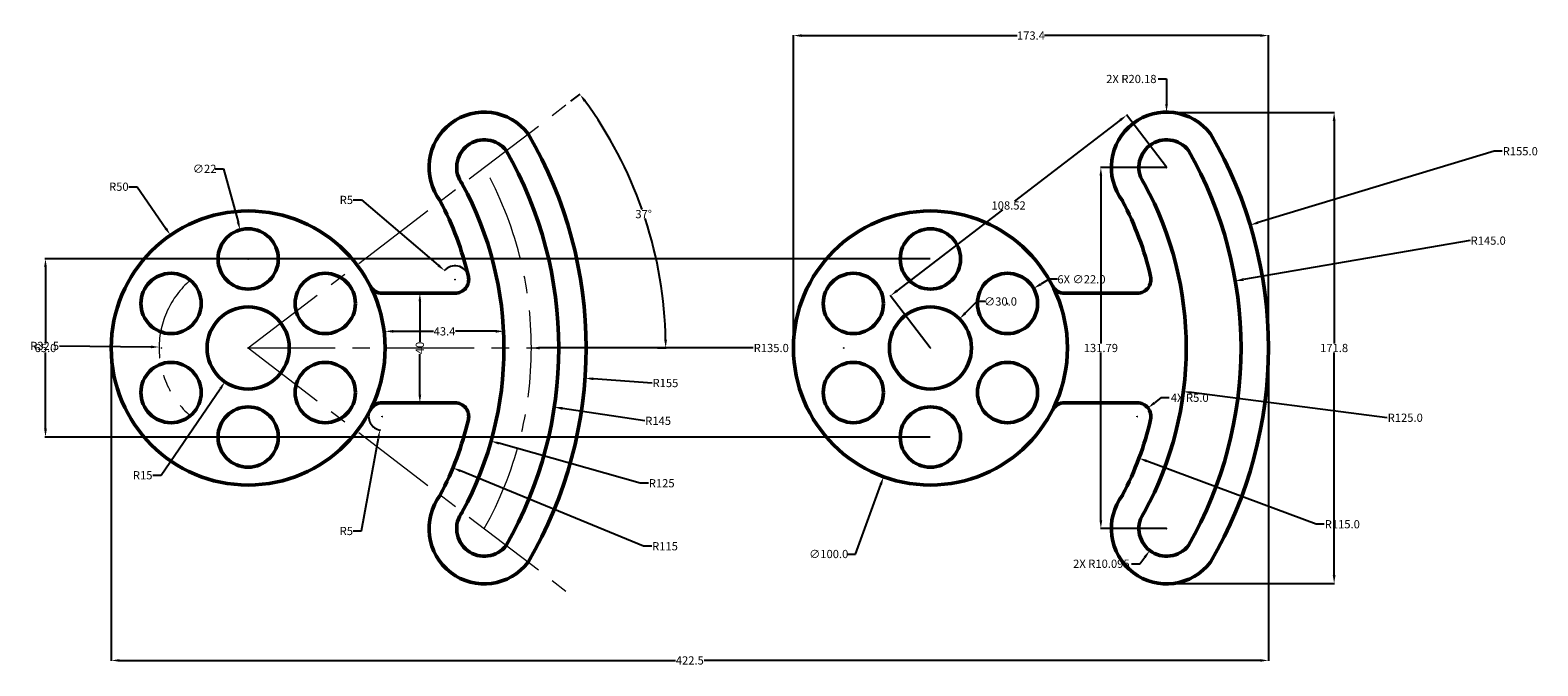
# Model space of a CAD drawing. Units: millimetres. Extents: x 51 to 601, y 33 to 265.
import ezdxf

# ---------------------------------------------------------------- set-up
doc = ezdxf.new("R2010")
doc.units = ezdxf.units.MM
doc.header["$MEASUREMENT"] = 0
doc.linetypes.add('CENTER', pattern=[50.8, 31.75, -6.35, 6.35, -6.35])
for name, color, linetype, lineweight in [('M-CNTR', 7, 'CENTER', 18), ('M-DIMS', 3, 'Continuous', 25), ('M-OUTL', 7, 'Continuous', 50)]:
    doc.layers.add(name, color=color, linetype=linetype, lineweight=lineweight)
doc.styles.get("Standard").update_dxf_attribs({"font": 'arial.ttf'})
doc.dimstyles.get("Standard").update_dxf_attribs({"dimtxt": 3, "dimasz": 3, "dimexe": 0.18, "dimexo": 0.0625, "dimgap": 0.09, "dimtad": 0, "dimtih": 1, "dimtoh": 1, "dimdec": 1, "dimdsep": 46, "dimtxsty": 'Standard', "dimcen": 0.09, "dimadec": 0, "dimazin": 0, "dimtfac": 1, "dimtdec": 1, "dimtofl": 0, "dimtmove": 0, "dimatfit": 3, "dimfxl": 1, "dimtolj": 1, "dimtzin": 0, "dimarcsym": 0})

# ---------------------------------------------------------------- blocks, each defined once
blk = doc.blocks.new('*D1')
at = {"layer": 'Defpoints', "color": 0, "transparency": 16777216}
for p in [(247.89, 238.72), (278.94, 181.6), (130.1, 148.71), (130.1, 148.71), (279.51, 148.71)]:
    blk.add_point(p, dxfattribs=at)
at = {"layer": 'M-DIMS', "color": 0, "lineweight": -2, "transparency": 16777216}
for p, q in [((247.93, 238.76), (251.36, 241.38)), ((279.57, 148.71), (282.72, 148.71))]:
    blk.add_line(p, q, dxfattribs=at)
for start, end in [(19.3385, 36.2591), (1.1276, 18.0507)]:
    blk.add_arc((130.1, 148.71), 152.44, start, end, dxfattribs=at)
at = {"layer": 'M-DIMS', "color": 0, "transparency": 16777216}
for points in [[(252.62, 238.57), (253.42, 239.16), (251.22, 241.27)], [(283.01, 151.71), (282.01, 151.7), (282.54, 148.71)]]:
    blk.add_solid(points, dxfattribs=at)
at = {"layer": 'M-DIMS', "color": 0, "transparency": 16777216, "insert": (274.49, 197.56), "char_height": 3, "attachment_point": 5}
blk.add_mtext('\\A1;37°', dxfattribs=at)
blk = doc.blocks.new('*D2')
at = {"layer": 'Defpoints', "color": 0, "transparency": 16777216}
for p in [(101.74, 189.89), (130.1, 148.71)]:
    blk.add_point(p, dxfattribs=at)
at = {"layer": 'M-DIMS', "color": 0, "lineweight": -2, "transparency": 16777216}
for p, q in [((86.56, 207.57), (89.56, 207.57)), ((89.56, 207.57), (100.03, 192.36)), ((130.01, 148.71), (130.19, 148.71)), ((130.1, 148.62), (130.1, 148.8))]:
    blk.add_line(p, q, dxfattribs=at)
at = {"layer": 'M-DIMS', "color": 0, "transparency": 16777216}
blk.add_solid([(100.45, 192.64), (99.62, 192.07), (101.74, 189.89)], dxfattribs=at)
at = {"layer": 'M-DIMS', "color": 0, "transparency": 16777216, "insert": (82.89, 207.57), "char_height": 3, "attachment_point": 5}
blk.add_mtext('\\A1;R50', dxfattribs=at)
blk = doc.blocks.new('*D3')
at = {"layer": 'Defpoints', "color": 0, "transparency": 16777216}
for p in [(127.18, 191.81), (133.01, 170.6)]:
    blk.add_point(p, dxfattribs=at)
at = {"layer": 'M-DIMS', "color": 0, "lineweight": -2, "transparency": 16777216}
for p, q in [((118.06, 214.1), (121.06, 214.1)), ((121.06, 214.1), (126.39, 194.71)), ((130.01, 181.21), (130.19, 181.21)), ((130.1, 181.12), (130.1, 181.3))]:
    blk.add_line(p, q, dxfattribs=at)
at = {"layer": 'M-DIMS', "color": 0, "transparency": 16777216}
blk.add_solid([(126.87, 194.84), (125.9, 194.57), (127.18, 191.81)], dxfattribs=at)
at = {"layer": 'M-DIMS', "color": 0, "transparency": 16777216, "insert": (114.2, 214.1), "char_height": 3, "attachment_point": 5}
blk.add_mtext('\\A1;∅22', dxfattribs=at)
blk = doc.blocks.new('*D4')
at = {"layer": 'Defpoints', "color": 0, "transparency": 16777216}
for p in [(130.1, 148.71), (121.62, 136.33)]:
    blk.add_point(p, dxfattribs=at)
at = {"layer": 'M-DIMS', "color": 0, "lineweight": -2, "transparency": 16777216}
for p, q in [((130.01, 148.71), (130.19, 148.71)), ((130.1, 148.62), (130.1, 148.8)), ((98.28, 102.26), (119.92, 133.86)), ((95.28, 102.26), (98.28, 102.26))]:
    blk.add_line(p, q, dxfattribs=at)
at = {"layer": 'M-DIMS', "color": 0, "transparency": 16777216}
blk.add_solid([(119.51, 134.14), (120.34, 133.57), (121.62, 136.33)], dxfattribs=at)
at = {"layer": 'M-DIMS', "color": 0, "transparency": 16777216, "insert": (91.6, 102.26), "char_height": 3, "attachment_point": 5}
blk.add_mtext('\\A1;R15', dxfattribs=at)
blk = doc.blocks.new('*D5')
at = {"layer": 'Defpoints', "color": 0, "transparency": 16777216}
for p in [(97.6, 149.06), (130.1, 148.71)]:
    blk.add_point(p, dxfattribs=at)
at = {"layer": 'M-DIMS', "color": 0, "lineweight": -2, "transparency": 16777216}
for p, q in [((61.21, 149.47), (94.6, 149.1)), ((130.01, 148.71), (130.19, 148.71)), ((130.1, 148.62), (130.1, 148.8))]:
    blk.add_line(p, q, dxfattribs=at)
at = {"layer": 'M-DIMS', "color": 0, "transparency": 16777216}
blk.add_solid([(94.6, 149.6), (94.59, 148.6), (97.6, 149.06)], dxfattribs=at)
at = {"layer": 'M-DIMS', "color": 0, "transparency": 16777216, "insert": (55.78, 149.47), "char_height": 3, "attachment_point": 5}
blk.add_mtext('\\A1;R32.5', dxfattribs=at)
blk = doc.blocks.new('*D6')
at = {"layer": 'Defpoints', "color": 0, "transparency": 16777216}
for p in [(192.35, 168.71), (192.35, 128.71), (192.78, 128.71)]:
    blk.add_point(p, dxfattribs=at)
at = {"layer": 'M-DIMS', "color": 0, "lineweight": -2, "transparency": 16777216}
for p, q in [((192.41, 168.71), (192.96, 168.71)), ((192.78, 165.71), (192.78, 151)), ((192.78, 131.71), (192.78, 146.41)), ((192.41, 128.71), (192.96, 128.71))]:
    blk.add_line(p, q, dxfattribs=at)
at = {"layer": 'M-DIMS', "color": 0, "transparency": 16777216}
for points in [[(192.28, 165.71), (193.28, 165.71), (192.78, 168.71)], [(192.28, 131.71), (193.28, 131.71), (192.78, 128.71)]]:
    blk.add_solid(points, dxfattribs=at)
at = {"layer": 'M-DIMS', "color": 0, "transparency": 16777216, "insert": (192.78, 148.71), "char_height": 3, "attachment_point": 5, "rotation": 90}
blk.add_mtext('\\A1;40', dxfattribs=at)
blk = doc.blocks.new('*D7')
at = {"layer": 'Defpoints', "color": 0, "transparency": 16777216}
for p in [(223.5, 154.79), (180.1, 148.71), (223.5, 148.71)]:
    blk.add_point(p, dxfattribs=at)
at = {"layer": 'M-DIMS', "color": 0, "lineweight": -2, "transparency": 16777216}
for p, q in [((180.1, 148.77), (180.1, 154.97)), ((183.1, 154.79), (197.75, 154.79)), ((220.5, 154.79), (205.84, 154.79)), ((223.5, 148.77), (223.5, 154.97))]:
    blk.add_line(p, q, dxfattribs=at)
at = {"layer": 'M-DIMS', "color": 0, "transparency": 16777216}
for points in [[(183.1, 155.29), (183.1, 154.29), (180.1, 154.79)], [(220.5, 155.29), (220.5, 154.29), (223.5, 154.79)]]:
    blk.add_solid(points, dxfattribs=at)
at = {"layer": 'M-DIMS', "color": 0, "transparency": 16777216, "insert": (201.8, 154.79), "char_height": 3, "attachment_point": 5}
blk.add_mtext('\\A1;43.4', dxfattribs=at)
blk = doc.blocks.new('*D8')
at = {"layer": 'Defpoints', "color": 0, "transparency": 16777216}
for p in [(179.08, 123.71), (178.19, 118.79)]:
    blk.add_point(p, dxfattribs=at)
at = {"layer": 'M-DIMS', "color": 0, "lineweight": -2, "transparency": 16777216}
for p, q in [((178.99, 123.71), (179.17, 123.71)), ((179.08, 123.62), (179.08, 123.8)), ((171.46, 81.93), (177.65, 115.84)), ((168.46, 81.93), (171.46, 81.93))]:
    blk.add_line(p, q, dxfattribs=at)
blk.add_arc((179.08, 123.71), 5, 153.6805, 261.7198, dxfattribs=at)
at = {"layer": 'M-DIMS', "color": 0, "transparency": 16777216}
blk.add_solid([(177.16, 115.93), (178.14, 115.75), (178.19, 118.79)], dxfattribs=at)
at = {"layer": 'M-DIMS', "color": 0, "transparency": 16777216, "insert": (165.94, 81.93), "char_height": 3, "attachment_point": 5}
blk.add_mtext('\\A1;R5', dxfattribs=at)
blk = doc.blocks.new('*D9')
at = {"layer": 'Defpoints', "color": 0, "transparency": 16777216}
for p in [(201.81, 176.94), (205.62, 173.71)]:
    blk.add_point(p, dxfattribs=at)
at = {"layer": 'M-DIMS', "color": 0, "lineweight": -2, "transparency": 16777216}
for p, q in [((168.47, 202.74), (171.47, 202.74)), ((171.47, 202.74), (199.52, 178.89)), ((205.53, 173.71), (205.71, 173.71)), ((205.62, 173.62), (205.62, 173.8))]:
    blk.add_line(p, q, dxfattribs=at)
blk.add_arc((205.62, 173.71), 5, 13.8528, 141.6868, dxfattribs=at)
at = {"layer": 'M-DIMS', "color": 0, "transparency": 16777216}
blk.add_solid([(199.85, 179.27), (199.2, 178.51), (201.81, 176.94)], dxfattribs=at)
at = {"layer": 'M-DIMS', "color": 0, "transparency": 16777216, "insert": (165.95, 202.74), "char_height": 3, "attachment_point": 5}
blk.add_mtext('\\A1;R5', dxfattribs=at)
blk = doc.blocks.new('*D10')
at = {"layer": 'Defpoints', "color": 0, "transparency": 16777216}
for p in [(98.5, 148.71), (204.85, 104.97)]:
    blk.add_point(p, dxfattribs=at)
at = {"layer": 'M-DIMS', "color": 0, "lineweight": -2, "transparency": 16777216}
for p, q in [((98.41, 148.71), (98.59, 148.71)), ((98.5, 148.62), (98.5, 148.8)), ((274.44, 76.36), (207.63, 103.83)), ((277.44, 76.36), (274.44, 76.36))]:
    blk.add_line(p, q, dxfattribs=at)
at = {"layer": 'M-DIMS', "color": 0, "transparency": 16777216}
blk.add_solid([(207.82, 104.29), (207.44, 103.37), (204.85, 104.97)], dxfattribs=at)
at = {"layer": 'M-DIMS', "color": 0, "transparency": 16777216, "insert": (282.29, 76.36), "char_height": 3, "attachment_point": 5}
blk.add_mtext('\\A1;R115', dxfattribs=at)
blk = doc.blocks.new('*D11')
at = {"layer": 'Defpoints', "color": 0, "transparency": 16777216}
for p in [(98.5, 148.71), (218.79, 114.73)]:
    blk.add_point(p, dxfattribs=at)
at = {"layer": 'M-DIMS', "color": 0, "lineweight": -2, "transparency": 16777216}
for p, q in [((98.41, 148.71), (98.59, 148.71)), ((98.5, 148.62), (98.5, 148.8)), ((273.23, 99.35), (221.68, 113.92)), ((276.23, 99.35), (273.23, 99.35))]:
    blk.add_line(p, q, dxfattribs=at)
at = {"layer": 'M-DIMS', "color": 0, "transparency": 16777216}
blk.add_solid([(221.81, 114.4), (221.54, 113.43), (218.79, 114.73)], dxfattribs=at)
at = {"layer": 'M-DIMS', "color": 0, "transparency": 16777216, "insert": (281.08, 99.35), "char_height": 3, "attachment_point": 5}
blk.add_mtext('\\A1;R125', dxfattribs=at)
blk = doc.blocks.new('*D12')
at = {"layer": 'Defpoints', "color": 0, "transparency": 16777216}
for p in [(98.5, 148.71), (241.88, 127.11)]:
    blk.add_point(p, dxfattribs=at)
at = {"layer": 'M-DIMS', "color": 0, "lineweight": -2, "transparency": 16777216}
for p, q in [((98.41, 148.71), (98.59, 148.71)), ((98.5, 148.62), (98.5, 148.8)), ((274.93, 122.13), (244.84, 126.67))]:
    blk.add_line(p, q, dxfattribs=at)
at = {"layer": 'M-DIMS', "color": 0, "transparency": 16777216}
blk.add_solid([(244.92, 127.16), (244.77, 126.17), (241.88, 127.11)], dxfattribs=at)
at = {"layer": 'M-DIMS', "color": 0, "transparency": 16777216, "insert": (279.78, 122.13), "char_height": 3, "attachment_point": 5}
blk.add_mtext('\\A1;R145', dxfattribs=at)
blk = doc.blocks.new('*D13')
at = {"layer": 'Defpoints', "color": 0, "transparency": 16777216}
for p in [(98.5, 148.71), (253.1, 137.68)]:
    blk.add_point(p, dxfattribs=at)
at = {"layer": 'M-DIMS', "color": 0, "lineweight": -2, "transparency": 16777216}
for p, q in [((98.41, 148.71), (98.59, 148.71)), ((98.5, 148.62), (98.5, 148.8)), ((277.6, 135.93), (256.09, 137.47))]:
    blk.add_line(p, q, dxfattribs=at)
at = {"layer": 'M-DIMS', "color": 0, "transparency": 16777216}
blk.add_solid([(256.13, 137.97), (256.06, 136.97), (253.1, 137.68)], dxfattribs=at)
at = {"layer": 'M-DIMS', "color": 0, "transparency": 16777216, "insert": (282.45, 135.93), "char_height": 3, "attachment_point": 5}
blk.add_mtext('\\A1;R155', dxfattribs=at)
blk = doc.blocks.new('FLANGE-SLOTTED-ARM')
at = {"transparency": 33554610}
for p, q in [((48.99, 20), (75.52, 20)), ((48.99, -20), (75.52, -20))]:
    blk.add_line(p, q, dxfattribs=at)
for centre, radius in [((0, 0), 50), ((0, 32.5), 11), ((-28.15, 16.25), 11), ((28.15, 16.25), 11), ((0, 0), 15), ((-28.15, -16.25), 11), ((28.15, -16.25), 11), ((0, -32.5), 11)]:
    blk.add_circle(centre, radius, dxfattribs=at)
for centre, radius, start, end in [((86.23, 65.89), 20.18, 37.3867, 217.3867), ((-31.6, 0), 155, 329.7241, 30.2759), ((86.23, 65.89), 10.1, 37.3867, 217.3867), ((-31.6, 0), 145, 330.2173, 29.7827), ((-31.6, 0), 125, 331.443, 28.557), ((-31.6, 0), 115, 13.1366, 27.7822), ((48.99, 25), 5, 207.0357, 270), ((75.52, 25), 5, 270, 13.1366), ((48.99, -25), 5, 90, 152.9643), ((75.52, -25), 5, 346.8634, 90), ((-31.6, 0), 115, 332.2178, 346.8634), ((86.23, -65.89), 20.18, 142.6133, 322.6133), ((86.23, -65.89), 10.1, 142.6133, 322.6133)]:
    blk.add_arc(centre, radius, start, end, dxfattribs=at)
blk = doc.blocks.new('*D15')
at = {"layer": 'Defpoints', "color": 0, "transparency": 16777216}
for p in [(502.59, 262.72), (329.19, 148.71), (502.59, 148.71)]:
    blk.add_point(p, dxfattribs=at)
at = {"layer": 'M-DIMS', "color": 0, "lineweight": -2, "transparency": 16777216}
for p, q in [((329.19, 148.77), (329.19, 262.9)), ((332.19, 262.72), (410.89, 262.72)), ((499.59, 262.72), (420.9, 262.72)), ((502.59, 148.77), (502.59, 262.9))]:
    blk.add_line(p, q, dxfattribs=at)
at = {"layer": 'M-DIMS', "color": 0, "transparency": 16777216}
for points in [[(332.19, 263.22), (332.19, 262.22), (329.19, 262.72)], [(499.59, 263.22), (499.59, 262.22), (502.59, 262.72)]]:
    blk.add_solid(points, dxfattribs=at)
at = {"layer": 'M-DIMS', "color": 0, "transparency": 16777216, "insert": (415.89, 262.72), "char_height": 3, "attachment_point": 5}
blk.add_mtext('\\A1;173.4', dxfattribs=at)
blk = doc.blocks.new('*D16')
at = {"layer": 'Defpoints', "color": 0, "transparency": 16777216}
for p in [(468.09, 234.6), (526.59, 234.6), (468.09, 62.81)]:
    blk.add_point(p, dxfattribs=at)
at = {"layer": 'M-DIMS', "color": 0, "lineweight": -2, "transparency": 16777216}
for p, q in [((468.16, 234.6), (526.77, 234.6)), ((526.59, 231.6), (526.59, 150.33)), ((526.59, 65.81), (526.59, 147.08)), ((468.16, 62.81), (526.77, 62.81))]:
    blk.add_line(p, q, dxfattribs=at)
at = {"layer": 'M-DIMS', "color": 0, "transparency": 16777216}
for points in [[(526.09, 231.6), (527.09, 231.6), (526.59, 234.6)], [(526.09, 65.81), (527.09, 65.81), (526.59, 62.81)]]:
    blk.add_solid(points, dxfattribs=at)
at = {"layer": 'M-DIMS', "color": 0, "transparency": 16777216, "insert": (526.59, 148.71), "char_height": 3, "attachment_point": 5}
blk.add_mtext('\\A1;171.8', dxfattribs=at)
blk = doc.blocks.new('*D17')
at = {"layer": 'Defpoints', "color": 0, "transparency": 16777216}
for p in [(80.1, 148.71), (502.59, 148.71), (502.59, 34.69)]:
    blk.add_point(p, dxfattribs=at)
at = {"layer": 'M-DIMS', "color": 0, "lineweight": -2, "transparency": 16777216}
for p, q in [((80.1, 148.64), (80.1, 34.51)), ((502.59, 148.64), (502.59, 34.51)), ((83.1, 34.69), (286.12, 34.69)), ((499.59, 34.69), (296.57, 34.69))]:
    blk.add_line(p, q, dxfattribs=at)
at = {"layer": 'M-DIMS', "color": 0, "transparency": 16777216}
for points in [[(83.1, 35.19), (83.1, 34.19), (80.1, 34.69)], [(499.59, 35.19), (499.59, 34.19), (502.59, 34.69)]]:
    blk.add_solid(points, dxfattribs=at)
at = {"layer": 'M-DIMS', "color": 0, "transparency": 16777216, "insert": (291.35, 34.69), "char_height": 3, "attachment_point": 5}
blk.add_mtext('\\A1;422.5', dxfattribs=at)
blk = doc.blocks.new('*D18')
at = {"layer": 'Defpoints', "color": 0, "transparency": 16777216}
for p in [(450.85, 233.67), (465.42, 214.6), (379.19, 148.71)]:
    blk.add_point(p, dxfattribs=at)
at = {"layer": 'M-DIMS', "color": 0, "lineweight": -2, "transparency": 16777216}
for p, q in [((448.47, 231.85), (409.86, 202.34)), ((465.38, 214.65), (450.74, 233.81)), ((367.01, 169.6), (405.61, 199.1)), ((379.16, 148.76), (364.51, 167.92))]:
    blk.add_line(p, q, dxfattribs=at)
at = {"layer": 'M-DIMS', "color": 0, "transparency": 16777216}
for points in [[(448.16, 232.24), (448.77, 231.45), (450.85, 233.67)], [(366.7, 169.99), (367.31, 169.2), (364.62, 167.77)]]:
    blk.add_solid(points, dxfattribs=at)
at = {"layer": 'M-DIMS', "color": 0, "transparency": 16777216, "insert": (407.74, 200.72), "char_height": 3, "attachment_point": 5}
blk.add_mtext('\\A1;108.52', dxfattribs=at)
blk = doc.blocks.new('*D19')
at = {"layer": 'Defpoints', "color": 0, "transparency": 16777216}
for p in [(56.1, 181.21), (379.19, 181.21), (379.19, 116.21)]:
    blk.add_point(p, dxfattribs=at)
at = {"layer": 'M-DIMS', "color": 0, "lineweight": -2, "transparency": 16777216}
for p, q in [((379.13, 181.21), (55.92, 181.21)), ((56.1, 178.21), (56.1, 150.33)), ((56.1, 119.21), (56.1, 147.08)), ((379.13, 116.21), (55.92, 116.21))]:
    blk.add_line(p, q, dxfattribs=at)
at = {"layer": 'M-DIMS', "color": 0, "transparency": 16777216}
for points in [[(55.6, 178.21), (56.6, 178.21), (56.1, 181.21)], [(55.6, 119.21), (56.6, 119.21), (56.1, 116.21)]]:
    blk.add_solid(points, dxfattribs=at)
at = {"layer": 'M-DIMS', "color": 0, "transparency": 16777216, "insert": (56.1, 148.71), "char_height": 3, "attachment_point": 5}
blk.add_mtext('\\A1;65.0', dxfattribs=at)
blk = doc.blocks.new('*D20')
at = {"layer": 'Defpoints', "color": 0, "transparency": 16777216}
for p in [(441.42, 214.6), (465.42, 214.6), (465.42, 82.81)]:
    blk.add_point(p, dxfattribs=at)
at = {"layer": 'M-DIMS', "color": 0, "lineweight": -2, "transparency": 16777216}
for p, q in [((465.36, 214.6), (441.24, 214.6)), ((441.42, 211.6), (441.42, 150.33)), ((441.42, 85.81), (441.42, 147.08)), ((465.36, 82.81), (441.24, 82.81))]:
    blk.add_line(p, q, dxfattribs=at)
at = {"layer": 'M-DIMS', "color": 0, "transparency": 16777216}
for points in [[(440.92, 211.6), (441.92, 211.6), (441.42, 214.6)], [(440.92, 85.81), (441.92, 85.81), (441.42, 82.81)]]:
    blk.add_solid(points, dxfattribs=at)
at = {"layer": 'M-DIMS', "color": 0, "transparency": 16777216, "insert": (441.42, 148.71), "char_height": 3, "attachment_point": 5}
blk.add_mtext('\\A1;131.79', dxfattribs=at)
blk = doc.blocks.new('*D21')
at = {"layer": 'Defpoints', "color": 0, "transparency": 16777216}
for p in [(98.5, 148.71), (233.5, 148.71)]:
    blk.add_point(p, dxfattribs=at)
at = {"layer": 'M-DIMS', "color": 0, "lineweight": -2, "transparency": 16777216}
for p, q in [((98.41, 148.71), (98.59, 148.71)), ((98.5, 148.62), (98.5, 148.8)), ((314.5, 148.71), (236.5, 148.71))]:
    blk.add_line(p, q, dxfattribs=at)
at = {"layer": 'M-DIMS', "color": 0, "transparency": 16777216}
blk.add_solid([(236.5, 149.21), (236.5, 148.21), (233.5, 148.71)], dxfattribs=at)
at = {"layer": 'M-DIMS', "color": 0, "transparency": 16777216, "insert": (321.08, 148.71), "char_height": 3, "attachment_point": 5}
blk.add_mtext('\\A1;R135.0', dxfattribs=at)
blk = doc.blocks.new('*D22')
at = {"layer": 'Defpoints', "color": 0, "transparency": 16777216}
for p in [(465.4, 234.78), (465.42, 214.6)]:
    blk.add_point(p, dxfattribs=at)
at = {"layer": 'M-DIMS', "color": 0, "lineweight": -2, "transparency": 16777216}
for p, q in [((462.39, 246.88), (465.39, 246.88)), ((465.39, 246.88), (465.4, 237.78)), ((465.42, 214.51), (465.42, 214.69)), ((465.33, 214.6), (465.51, 214.6))]:
    blk.add_line(p, q, dxfattribs=at)
at = {"layer": 'M-DIMS', "color": 0, "transparency": 16777216}
blk.add_solid([(465.9, 237.78), (464.9, 237.78), (465.4, 234.78)], dxfattribs=at)
at = {"layer": 'M-DIMS', "color": 0, "transparency": 16777216, "insert": (452.55, 246.88), "char_height": 3, "attachment_point": 5}
blk.add_mtext('\\A1;2X R20.18', dxfattribs=at)
blk = doc.blocks.new('*D23')
at = {"layer": 'Defpoints', "color": 0, "transparency": 16777216}
for p in [(465.42, 82.81), (459.29, 74.79)]:
    blk.add_point(p, dxfattribs=at)
at = {"layer": 'M-DIMS', "color": 0, "lineweight": -2, "transparency": 16777216}
for p, q in [((465.33, 82.81), (465.51, 82.81)), ((465.42, 82.72), (465.42, 82.9)), ((455.61, 69.98), (457.47, 72.41)), ((452.61, 69.98), (455.61, 69.98))]:
    blk.add_line(p, q, dxfattribs=at)
at = {"layer": 'M-DIMS', "color": 0, "transparency": 16777216}
blk.add_solid([(457.07, 72.71), (457.87, 72.1), (459.29, 74.79)], dxfattribs=at)
at = {"layer": 'M-DIMS', "color": 0, "transparency": 16777216, "insert": (441.6, 69.98), "char_height": 3, "attachment_point": 5}
blk.add_mtext('\\A1;2X R10.095', dxfattribs=at)
blk = doc.blocks.new('*D24')
at = {"layer": 'Defpoints', "color": 0, "transparency": 16777216}
for p in [(495.96, 193.59), (347.59, 148.71)]:
    blk.add_point(p, dxfattribs=at)
at = {"layer": 'M-DIMS', "color": 0, "lineweight": -2, "transparency": 16777216}
for p, q in [((584.97, 220.51), (498.83, 194.46)), ((587.97, 220.51), (584.97, 220.51)), ((347.5, 148.71), (347.68, 148.71)), ((347.59, 148.62), (347.59, 148.8))]:
    blk.add_line(p, q, dxfattribs=at)
at = {"layer": 'M-DIMS', "color": 0, "transparency": 16777216}
blk.add_solid([(498.68, 194.93), (498.97, 193.98), (495.96, 193.59)], dxfattribs=at)
at = {"layer": 'M-DIMS', "color": 0, "transparency": 16777216, "insert": (594.55, 220.51), "char_height": 3, "attachment_point": 5}
blk.add_mtext('\\A1;R155.0', dxfattribs=at)
blk = doc.blocks.new('*D25')
at = {"layer": 'Defpoints', "color": 0, "transparency": 16777216}
for p in [(490.51, 173.2), (347.59, 148.71)]:
    blk.add_point(p, dxfattribs=at)
at = {"layer": 'M-DIMS', "color": 0, "lineweight": -2, "transparency": 16777216}
for p, q in [((576.26, 187.89), (493.47, 173.71)), ((347.5, 148.71), (347.68, 148.71)), ((347.59, 148.62), (347.59, 148.8))]:
    blk.add_line(p, q, dxfattribs=at)
at = {"layer": 'M-DIMS', "color": 0, "transparency": 16777216}
blk.add_solid([(493.38, 174.2), (493.55, 173.21), (490.51, 173.2)], dxfattribs=at)
at = {"layer": 'M-DIMS', "color": 0, "transparency": 16777216, "insert": (582.84, 187.89), "char_height": 3, "attachment_point": 5}
blk.add_mtext('\\A1;R145.0', dxfattribs=at)
blk = doc.blocks.new('*D26')
at = {"layer": 'Defpoints', "color": 0, "transparency": 16777216}
for p in [(347.59, 148.71), (471.58, 132.8)]:
    blk.add_point(p, dxfattribs=at)
at = {"layer": 'M-DIMS', "color": 0, "lineweight": -2, "transparency": 16777216}
for p, q in [((347.5, 148.71), (347.68, 148.71)), ((347.59, 148.62), (347.59, 148.8)), ((545.97, 123.26), (474.55, 132.42))]:
    blk.add_line(p, q, dxfattribs=at)
at = {"layer": 'M-DIMS', "color": 0, "transparency": 16777216}
blk.add_solid([(474.62, 132.91), (474.49, 131.92), (471.58, 132.8)], dxfattribs=at)
at = {"layer": 'M-DIMS', "color": 0, "transparency": 16777216, "insert": (552.55, 123.26), "char_height": 3, "attachment_point": 5}
blk.add_mtext('\\A1;R125.0', dxfattribs=at)
blk = doc.blocks.new('*D27')
at = {"layer": 'Defpoints', "color": 0, "transparency": 16777216}
for p in [(347.59, 148.71), (455.34, 108.51)]:
    blk.add_point(p, dxfattribs=at)
at = {"layer": 'M-DIMS', "color": 0, "lineweight": -2, "transparency": 16777216}
for p, q in [((347.5, 148.71), (347.68, 148.71)), ((347.59, 148.62), (347.59, 148.8)), ((519.99, 84.39), (458.15, 107.46)), ((522.99, 84.39), (519.99, 84.39))]:
    blk.add_line(p, q, dxfattribs=at)
at = {"layer": 'M-DIMS', "color": 0, "transparency": 16777216}
blk.add_solid([(458.33, 107.93), (457.98, 106.99), (455.34, 108.51)], dxfattribs=at)
at = {"layer": 'M-DIMS', "color": 0, "transparency": 16777216, "insert": (529.57, 84.39), "char_height": 3, "attachment_point": 5}
blk.add_mtext('\\A1;R115.0', dxfattribs=at)
blk = doc.blocks.new('*D28')
at = {"layer": 'Defpoints', "color": 0, "transparency": 16777216}
for p in [(458.63, 126.81), (454.72, 123.71)]:
    blk.add_point(p, dxfattribs=at)
at = {"layer": 'M-DIMS', "color": 0, "lineweight": -2, "transparency": 16777216}
for p, q in [((463.33, 130.54), (460.98, 128.68)), ((466.33, 130.54), (463.33, 130.54)), ((454.63, 123.71), (454.81, 123.71)), ((454.72, 123.62), (454.72, 123.8))]:
    blk.add_line(p, q, dxfattribs=at)
at = {"layer": 'M-DIMS', "color": 0, "transparency": 16777216}
blk.add_solid([(460.67, 129.07), (461.29, 128.29), (458.63, 126.81)], dxfattribs=at)
at = {"layer": 'M-DIMS', "color": 0, "transparency": 16777216, "insert": (473.87, 130.54), "char_height": 3, "attachment_point": 5}
blk.add_mtext('\\A1;4X R5.0', dxfattribs=at)
blk = doc.blocks.new('*D29')
at = {"layer": 'Defpoints', "color": 0, "transparency": 16777216}
for p in [(396.3, 195.69), (362.09, 101.72)]:
    blk.add_point(p, dxfattribs=at)
at = {"layer": 'M-DIMS', "color": 0, "lineweight": -2, "transparency": 16777216}
for p, q in [((379.1, 148.71), (379.28, 148.71)), ((379.19, 148.62), (379.19, 148.8)), ((351.83, 73.53), (361.07, 98.9)), ((348.83, 73.53), (351.83, 73.53))]:
    blk.add_line(p, q, dxfattribs=at)
at = {"layer": 'M-DIMS', "color": 0, "transparency": 16777216}
blk.add_solid([(360.6, 99.07), (361.54, 98.73), (362.09, 101.72)], dxfattribs=at)
at = {"layer": 'M-DIMS', "color": 0, "transparency": 16777216, "insert": (342.06, 73.53), "char_height": 3, "attachment_point": 5}
blk.add_mtext('\\A1;∅100.0', dxfattribs=at)
blk = doc.blocks.new('*D30')
at = {"layer": 'Defpoints', "color": 0, "transparency": 16777216}
for p in [(389.8, 159.31), (368.59, 138.1)]:
    blk.add_point(p, dxfattribs=at)
at = {"layer": 'M-DIMS', "color": 0, "lineweight": -2, "transparency": 16777216}
for p, q in [((396.17, 165.68), (391.92, 161.43)), ((399.17, 165.68), (396.17, 165.68)), ((379.1, 148.71), (379.28, 148.71)), ((379.19, 148.62), (379.19, 148.8))]:
    blk.add_line(p, q, dxfattribs=at)
at = {"layer": 'M-DIMS', "color": 0, "transparency": 16777216}
blk.add_solid([(391.57, 161.79), (392.28, 161.08), (389.8, 159.31)], dxfattribs=at)
at = {"layer": 'M-DIMS', "color": 0, "transparency": 16777216, "insert": (404.78, 165.68), "char_height": 3, "attachment_point": 5}
blk.add_mtext('\\A1;∅30.0', dxfattribs=at)
blk = doc.blocks.new('*D31')
at = {"layer": 'Defpoints', "color": 0, "transparency": 16777216}
for p in [(416.86, 170.46), (397.82, 159.45)]:
    blk.add_point(p, dxfattribs=at)
at = {"layer": 'M-DIMS', "color": 0, "lineweight": -2, "transparency": 16777216}
for p, q in [((422.58, 173.77), (419.46, 171.97)), ((425.58, 173.77), (422.58, 173.77)), ((407.25, 164.96), (407.43, 164.96)), ((407.34, 164.87), (407.34, 165.05))]:
    blk.add_line(p, q, dxfattribs=at)
at = {"layer": 'M-DIMS', "color": 0, "transparency": 16777216}
blk.add_solid([(419.21, 172.4), (419.71, 171.53), (416.86, 170.46)], dxfattribs=at)
at = {"layer": 'M-DIMS', "color": 0, "transparency": 16777216, "insert": (434.34, 173.77), "char_height": 3, "attachment_point": 5}
blk.add_mtext('\\A1;6X ∅22.0', dxfattribs=at)

msp = doc.modelspace()

# ---------------------------------------------------------------- linework, layer by layer
at = {"layer": 'M-CNTR'}
for q in [(247.8851, 238.7197), (247.8851, 58.6916), (279.5056, 148.7057)]:
    msp.add_line((130.0951, 148.7057), q, dxfattribs=at)
for centre, radius, start, end in [((98.4951, 148.7057), 135, 330.784277, 29.215723), ((130.0951, 148.7057), 32.5, 130.513805, 229.486195)]:
    msp.add_arc(centre, radius, start, end, dxfattribs=at)

# ---------------------------------------------------------------- block references
at = {"layer": 'M-OUTL', "transparency": 33554610}
for p in [(130.0951, 148.7057), (379.1949, 148.7057)]:
    msp.add_blockref('FLANGE-SLOTTED-ARM', p, dxfattribs=at)

# ---------------------------------------------------------------- dimensions: what is measured, and where the dimension line sits
at = {"layer": 'M-DIMS', "transparency": 33554610}
for base, p1, p2, override, picture, middle in [((502.5949, 262.7197), (329.1949, 148.7057), (502.5949, 148.7057), {"dimdec": 1, "dimlfac": 1, "dimrnd": 0, "dimzin": 0, "dimdsep": 46, "dimlunit": 2}, '*D15', (415.8949, 262.7197)), ((223.4951, 154.7941), (180.0951, 148.7057), (223.4951, 148.7057), {"dimclrd": 0, "dimclre": 0, "dimclrt": 0}, '*D7', (201.7951, 154.7941)), ((502.5949, 34.6916), (80.0951, 148.7057), (502.5949, 148.7057), {"dimdec": 1, "dimlfac": 1, "dimrnd": 0, "dimzin": 0, "dimdsep": 46, "dimlunit": 2}, '*D17', (291.345, 34.6916))]:
    dim = msp.add_linear_dim(base=base, p1=p1, p2=p2, dimstyle='Standard', override=override, dxfattribs=at)
    dim.commit()
    dim.dimension.update_dxf_attribs({"geometry": picture, "text_midpoint": middle})
for center, mpoint, override, picture, middle in [((465.4213, 214.599), (465.4, 234.7773), {"dimdec": 2, "dimlfac": 1, "dimrnd": 0, "dimzin": 0, "dimdsep": 46, "dimlunit": 2}, '*D22', (452.5483, 246.8843)), ((465.4213, 82.8123), (459.2918, 74.7907), {"dimdec": 3, "dimlfac": 1, "dimrnd": 0, "dimzin": 0, "dimdsep": 46, "dimlunit": 2}, '*D23', (441.6015, 69.9778))]:
    dim = msp.add_radius_dim(center=center, mpoint=mpoint, text='2X <>', dimstyle='Standard', override=override, dxfattribs=at)
    dim.commit()
    dim.dimension.update_dxf_attribs({"geometry": picture, "text_midpoint": middle, "dimtype": 164})
dim = msp.add_angular_dim_2l(base=(278.9445, 181.6019), line1=((130.0951, 148.7057), (247.8851, 238.7197)), line2=((130.0951, 148.7057), (279.5056, 148.7057)), dimstyle='Standard', override={"dimclrd": 0, "dimclre": 0, "dimclrt": 0}, dxfattribs=at)
dim.commit()
dim.dimension.update_dxf_attribs({"geometry": '*D1', "text_midpoint": (274.4946, 197.5635)})
for base, p1, p2, angle, override, picture, middle in [((450.8487, 233.6684), (379.1949, 148.7057), (465.4213, 214.599), 37.386715, {"dimdec": 2, "dimlfac": 1, "dimrnd": 0, "dimzin": 0, "dimdsep": 46, "dimlunit": 2}, '*D18', (407.7355, 200.7217)), ((526.5949, 234.5995), (468.0947, 62.8118), (468.0947, 234.5995), 90, {"dimdec": 1, "dimlfac": 1, "dimrnd": 0, "dimzin": 0, "dimdsep": 46, "dimlunit": 2}, '*D16', (526.5949, 148.7057)), ((441.4213, 214.599), (465.4213, 82.8123), (465.4213, 214.599), 90, {"dimdec": 2, "dimlfac": 1, "dimrnd": 0, "dimzin": 0, "dimdsep": 46, "dimlunit": 2}, '*D20', (441.4213, 148.7057)), ((56.0951, 181.2057), (379.1949, 116.2057), (379.1949, 181.2057), 90, {"dimdec": 1, "dimlfac": 1, "dimrnd": 0, "dimzin": 0, "dimdsep": 46, "dimlunit": 2}, '*D19', (56.0951, 148.7057))]:
    dim = msp.add_linear_dim(base=base, p1=p1, p2=p2, angle=angle, dimstyle='Standard', override=override, dxfattribs=at)
    dim.commit()
    dim.dimension.update_dxf_attribs({"geometry": picture, "text_midpoint": middle})
for center, mpoint, override, picture, middle in [((347.5949, 148.7057), (495.955, 193.5864), {"dimdec": 1, "dimlfac": 1, "dimrnd": 0, "dimzin": 0, "dimdsep": 46, "dimlunit": 2}, '*D24', (594.5533, 220.5148)), ((130.0951, 148.7057), (101.7364, 189.8856), {"dimclrd": 0, "dimclre": 0, "dimclrt": 0}, '*D2', (82.8903, 207.5677)), ((205.6165, 173.7057), (201.8074, 176.9447), {"dimclrd": 0, "dimclre": 0, "dimclrt": 0}, '*D9', (165.9478, 202.7436)), ((347.5949, 148.7057), (490.5113, 173.1985), {"dimdec": 1, "dimlfac": 1, "dimrnd": 0, "dimzin": 0, "dimdsep": 46, "dimlunit": 2}, '*D25', (576.2612, 187.8942)), ((130.0951, 148.7057), (97.5971, 149.0646), {"dimclrd": 0, "dimclre": 0, "dimclrt": 0}, '*D5', (61.2125, 149.4666)), ((130.0951, 148.7057), (121.6186, 136.3303), {"dimclrd": 0, "dimclre": 0, "dimclrt": 0}, '*D4', (91.5961, 102.2594)), ((98.4951, 148.7057), (233.4951, 148.706), {"dimdec": 1, "dimlfac": 1, "dimrnd": 0, "dimzin": 0, "dimdsep": 46, "dimlunit": 2}, '*D21', (314.4951, 148.7062)), ((98.4951, 148.7057), (204.8544, 104.9713), {"dimclrd": 0, "dimclre": 0, "dimclrt": 0}, '*D10', (282.2946, 76.3566)), ((98.4951, 148.7057), (218.7894, 114.7311), {"dimclrd": 0, "dimclre": 0, "dimclrt": 0}, '*D11', (281.0832, 99.355)), ((98.4951, 148.7057), (241.8782, 127.1125), {"dimclrd": 0, "dimclre": 0, "dimclrt": 0}, '*D12', (274.9321, 122.1346)), ((98.4951, 148.7057), (253.1025, 137.6804), {"dimclrd": 0, "dimclre": 0, "dimclrt": 0}, '*D13', (277.5972, 135.9336)), ((347.5949, 148.7057), (471.5789, 132.8001), {"dimdec": 1, "dimlfac": 1, "dimrnd": 0, "dimzin": 0, "dimdsep": 46, "dimlunit": 2}, '*D26', (545.9692, 123.2568)), ((347.5949, 148.7057), (455.3407, 108.5081), {"dimdec": 1, "dimlfac": 1, "dimrnd": 0, "dimzin": 0, "dimdsep": 46, "dimlunit": 2}, '*D27', (529.5704, 84.3896)), ((179.0849, 123.7057), (178.1872, 118.7869), {"dimclrd": 0, "dimclre": 0, "dimclrt": 0}, '*D8', (165.9397, 81.9256))]:
    dim = msp.add_radius_dim(center=center, mpoint=mpoint, dimstyle='Standard', override=override, dxfattribs=at)
    dim.commit()
    dim.dimension.update_dxf_attribs({"geometry": picture, "text_midpoint": middle, "dimtype": 164})
for p1, p2, override, picture, middle in [((133.0093, 170.5987), (127.1808, 191.8126), {"dimclrd": 0, "dimclre": 0, "dimclrt": 0}, '*D3', (114.2008, 214.1041)), ((396.2956, 195.6904), (362.0943, 101.7209), {"dimdec": 1, "dimlfac": 1, "dimrnd": 0, "dimzin": 0, "dimdsep": 46, "dimlunit": 2}, '*D29', (342.0553, 73.53)), ((368.5885, 138.0989), (389.8014, 159.3124), {"dimdec": 1, "dimlfac": 1, "dimrnd": 0, "dimzin": 0, "dimdsep": 46, "dimlunit": 2}, '*D30', (404.7785, 165.6764))]:
    dim = msp.add_diameter_dim_2p(p1=p1, p2=p2, dimstyle='Standard', override=override, dxfattribs=at)
    dim.commit()
    dim.dimension.update_dxf_attribs({"geometry": picture, "text_midpoint": middle, "dimtype": 163})
dim = msp.add_diameter_dim_2p(p1=(397.8189, 159.448), p2=(416.8626, 170.4633), text='6X <>', dimstyle='Standard', override={"dimdec": 1, "dimlfac": 1, "dimrnd": 0, "dimzin": 0, "dimdsep": 46, "dimlunit": 2}, dxfattribs=at)
dim.commit()
dim.dimension.update_dxf_attribs({"geometry": '*D31', "text_midpoint": (434.3404, 173.7679), "dimtype": 163})
dim = msp.add_linear_dim(base=(192.7807, 128.7057), p1=(192.3507, 168.7057), p2=(192.3507, 128.7057), angle=90, dimstyle='Standard', override={"dimclrd": 0, "dimclre": 0, "dimclrt": 0}, dxfattribs=at)
dim.commit()
dim.dimension.update_dxf_attribs({"geometry": '*D6', "text_midpoint": (192.7807, 148.7057), "text_rotation": 90})
dim = msp.add_radius_dim(center=(454.7164, 123.7057), mpoint=(458.6329, 126.8139), text='4X <>', dimstyle='Standard', override={"dimdec": 1, "dimlfac": 1, "dimrnd": 0, "dimzin": 0, "dimdsep": 46, "dimlunit": 2}, dxfattribs=at)
dim.commit()
dim.dimension.update_dxf_attribs({"geometry": '*D28', "text_midpoint": (473.8674, 130.5438)})

doc.saveas('drawing.dxf')
